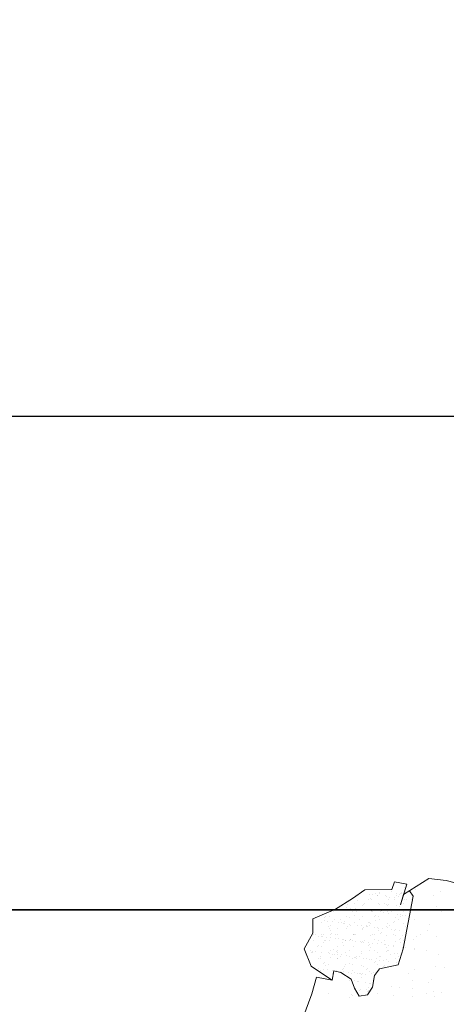
# Model space of a CAD drawing. Units: inches. Extents: x 1986 to 21484, y -1816 to 2016.
# Tile 35 of 85: x 2149 to 2160, y 1898 to 1924. Entities that reach past the tile are written whole.
import ezdxf

# ---------------------------------------------------------------- set-up
doc = ezdxf.new("R2010")
doc.units = ezdxf.units.IN
for name, color, linetype, lineweight in [('A-ANNO-DIMS', 2, 'Continuous', 18), ('C-PROP', 7, 'Continuous', 35), ('L-PLNT', 84, 'Continuous', 13)]:
    doc.layers.add(name, color=color, linetype=linetype, lineweight=lineweight)
doc.styles.get("Standard").update_dxf_attribs({"font": 'arial.ttf'})
doc.dimstyles.new('ISO-25', dxfattribs={"dimtxt": 8, "dimasz": 2.5, "dimexe": 1.25, "dimexo": 0.625, "dimtad": 1, "dimdec": 1, "dimlunit": 3, "dimtxsty": 'Standard', "dimcen": 2.5, "dimadec": 0, "dimazin": 0, "dimtfac": 1, "dimtdec": 1, "dimtmove": 0, "dimatfit": 3, "dimfxl": 1, "dimarcsym": 0})

# ---------------------------------------------------------------- blocks, each defined once
blk = doc.blocks.new('*D1')
at = {"layer": 'A-ANNO-DIMS', "color": 0, "lineweight": -2, "transparency": 16777216}
for p, q in [((2042.312, 1901.377), (2042.312, 1914.655)), ((2402.312, 1901.377), (2402.312, 1914.655)), ((2044.812, 1913.405), (2399.812, 1913.405))]:
    blk.add_line(p, q, dxfattribs=at)
at = {"layer": 'A-ANNO-DIMS', "color": 0, "transparency": 16777216}
for points in [[(2044.812, 1913.821), (2044.812, 1912.988), (2042.312, 1913.405)], [(2399.812, 1913.821), (2399.812, 1912.988), (2402.312, 1913.405)]]:
    blk.add_solid(points, dxfattribs=at)
at = {"layer": 'Defpoints', "color": 0, "transparency": 16777216}
for p in [(2402.312, 1913.405), (2042.312, 1900.752), (2402.312, 1900.752)]:
    blk.add_point(p, dxfattribs=at)
at = {"layer": 'A-ANNO-DIMS', "color": 0, "transparency": 16777216, "insert": (2222.312, 1918.117), "char_height": 8, "attachment_point": 5}
blk.add_mtext("30'", dxfattribs=at)
blk = doc.blocks.new('PLANT-SHRUB')
for p, q in [((2158.177, 1901.273), (2158.24, 1901.471)), ((2158.24, 1901.471), (2158.553, 1901.409)), ((2158.553, 1901.409), (2158.396, 1900.877)), ((2158.474, 1901.143), (2159.119, 1901.558)), ((2159.119, 1901.558), (2159.568, 1901.506)), ((2159.119, 1901.558), (2159.119, 1901.558)), ((2159.568, 1901.506), (2159.797, 1901.443)), ((2157.165, 1901.044), (2157.478, 1901.263)), ((2157.478, 1901.263), (2158.177, 1901.273)), ((2157.753, 1901.169), (2157.753, 1901.169)), ((2157.862, 1901.187), (2157.862, 1901.187)), ((2157.862, 1901.159), (2157.862, 1901.159)), ((2158.166, 1901.222), (2158.166, 1901.222)), ((2158.294, 1901.171), (2158.294, 1901.171)), ((2158.36, 1901.158), (2158.36, 1901.158)), ((2158.393, 1901.174), (2158.393, 1901.174)), ((2158.412, 1901.172), (2158.412, 1901.172)), ((2158.423, 1901.201), (2158.423, 1901.201)), ((2158.497, 1901.332), (2158.497, 1901.332)), ((2158.716, 1901.103), (2158.627, 1901.241)), ((2158.791, 1901.264), (2158.791, 1901.264)), ((2159.411, 1901.22), (2159.411, 1901.22)), ((2156.726, 1900.772), (2157.165, 1901.044)), ((2156.98, 1900.915), (2156.98, 1900.915)), ((2157.204, 1900.902), (2157.204, 1900.902)), ((2157.285, 1900.982), (2157.285, 1900.982)), ((2157.478, 1900.914), (2157.478, 1900.914)), ((2157.585, 1901.014), (2157.585, 1901.014)), ((2157.596, 1901.148), (2157.596, 1901.148)), ((2157.614, 1901.041), (2157.614, 1901.041)), ((2157.659, 1901.027), (2157.659, 1901.027)), ((2157.679, 1901.137), (2157.679, 1901.137)), ((2157.795, 1901.116), (2157.795, 1901.116)), ((2157.809, 1901.12), (2157.809, 1901.12)), ((2157.828, 1900.91), (2157.828, 1900.91)), ((2157.976, 1900.913), (2157.976, 1900.913)), ((2157.998, 1901.115), (2157.998, 1901.115)), ((2158.026, 1901.091), (2158.026, 1901.091)), ((2158.078, 1901.022), (2158.078, 1901.022)), ((2158.11, 1901.08), (2158.11, 1901.08)), ((2158.234, 1901.028), (2158.234, 1901.028)), ((2158.24, 1901.063), (2158.24, 1901.063)), ((2158.293, 1901.115), (2158.293, 1901.115)), ((2158.338, 1901.104), (2158.338, 1901.104)), ((2158.396, 1900.877), (2158.474, 1901.143)), ((2158.457, 1901.035), (2158.457, 1901.035)), ((2158.46, 1899.75), (2158.716, 1901.103)), ((2158.474, 1900.912), (2158.474, 1900.912)), ((2158.487, 1901.024), (2158.487, 1901.024)), ((2158.54, 1901.024), (2158.54, 1901.024)), ((2158.67, 1901.007), (2158.67, 1901.007)), ((2159.242, 1901.112), (2159.242, 1901.112)), ((2156.152, 1900.522), (2156.726, 1900.772)), ((2156.617, 1900.709), (2156.617, 1900.709)), ((2156.67, 1900.717), (2156.67, 1900.717)), ((2156.737, 1900.76), (2156.737, 1900.76)), ((2156.808, 1900.732), (2156.808, 1900.732)), ((2157.018, 1900.81), (2157.018, 1900.81)), ((2157.025, 1900.882), (2157.025, 1900.882)), ((2157.102, 1900.799), (2157.102, 1900.799)), ((2157.168, 1900.716), (2157.168, 1900.716)), ((2157.217, 1900.734), (2157.217, 1900.734)), ((2157.231, 1900.782), (2157.231, 1900.782)), ((2157.235, 1900.759), (2157.235, 1900.759)), ((2157.257, 1900.714), (2157.257, 1900.714)), ((2157.287, 1900.741), (2157.287, 1900.741)), ((2157.426, 1900.868), (2157.426, 1900.868)), ((2157.443, 1900.877), (2157.443, 1900.877)), ((2157.449, 1900.753), (2157.449, 1900.753)), ((2157.532, 1900.742), (2157.532, 1900.742)), ((2157.649, 1900.719), (2157.649, 1900.719)), ((2157.662, 1900.725), (2157.662, 1900.725)), ((2157.666, 1900.715), (2157.666, 1900.715)), ((2157.733, 1900.758), (2157.733, 1900.758)), ((2157.852, 1900.879), (2157.852, 1900.879)), ((2157.879, 1900.697), (2157.879, 1900.697)), ((2157.906, 1900.728), (2157.906, 1900.728)), ((2157.941, 1900.74), (2157.941, 1900.74)), ((2157.962, 1900.686), (2157.962, 1900.686)), ((2158.036, 1900.883), (2158.036, 1900.883)), ((2158.065, 1900.874), (2158.065, 1900.874)), ((2158.068, 1900.714), (2158.068, 1900.714)), ((2158.092, 1900.669), (2158.092, 1900.669)), ((2158.095, 1900.901), (2158.095, 1900.901)), ((2158.163, 1900.714), (2158.163, 1900.714)), ((2158.231, 1900.757), (2158.231, 1900.757)), ((2158.284, 1900.863), (2158.284, 1900.863)), ((2158.284, 1900.863), (2158.284, 1900.863)), ((2158.361, 1900.84), (2158.361, 1900.84)), ((2158.477, 1900.715), (2158.477, 1900.715)), ((2158.546, 1900.734), (2158.546, 1900.734)), ((2158.575, 1900.761), (2158.575, 1900.761)), ((2158.904, 1900.769), (2158.904, 1900.769)), ((2159.112, 1900.741), (2159.112, 1900.741)), ((2159.33, 1900.85), (2159.33, 1900.85)), ((2159.437, 1900.699), (2159.437, 1900.699)), ((2159.54, 1900.753), (2159.54, 1900.753)), ((2156.152, 1900.157), (2156.152, 1900.522)), ((2156.38, 1900.43), (2156.38, 1900.43)), ((2156.441, 1900.472), (2156.441, 1900.472)), ((2156.449, 1900.554), (2156.449, 1900.554)), ((2156.478, 1900.581), (2156.478, 1900.581)), ((2156.524, 1900.461), (2156.524, 1900.461)), ((2156.583, 1900.59), (2156.583, 1900.59)), ((2156.654, 1900.444), (2156.654, 1900.444)), ((2156.697, 1900.502), (2156.697, 1900.502)), ((2156.798, 1900.424), (2156.798, 1900.424)), ((2156.851, 1900.514), (2156.851, 1900.514)), ((2156.871, 1900.416), (2156.871, 1900.416)), ((2156.929, 1900.414), (2156.929, 1900.414)), ((2156.954, 1900.405), (2156.954, 1900.405)), ((2156.959, 1900.441), (2156.959, 1900.441)), ((2157.014, 1900.574), (2157.014, 1900.574)), ((2157.098, 1900.568), (2157.098, 1900.568)), ((2157.206, 1900.61), (2157.206, 1900.61)), ((2157.207, 1900.426), (2157.207, 1900.426)), ((2157.349, 1900.513), (2157.349, 1900.513)), ((2157.433, 1900.569), (2157.433, 1900.569)), ((2157.579, 1900.428), (2157.579, 1900.428)), ((2157.593, 1900.421), (2157.593, 1900.421)), ((2157.639, 1900.411), (2157.639, 1900.411)), ((2157.738, 1900.574), (2157.738, 1900.574)), ((2157.743, 1900.489), (2157.743, 1900.489)), ((2157.767, 1900.601), (2157.767, 1900.601)), ((2157.842, 1900.571), (2157.842, 1900.571)), ((2157.847, 1900.513), (2157.847, 1900.513)), ((2158.057, 1900.405), (2158.057, 1900.405)), ((2158.218, 1900.433), (2158.218, 1900.433)), ((2158.248, 1900.46), (2158.248, 1900.46)), ((2158.274, 1900.555), (2158.274, 1900.555)), ((2158.309, 1900.64), (2158.309, 1900.64)), ((2158.344, 1900.512), (2158.344, 1900.512)), ((2158.387, 1900.588), (2158.387, 1900.588)), ((2158.392, 1900.629), (2158.392, 1900.629)), ((2158.45, 1900.608), (2158.45, 1900.608)), ((2158.466, 1900.407), (2158.466, 1900.407)), ((2158.522, 1900.612), (2158.522, 1900.612)), ((2158.766, 1900.494), (2158.766, 1900.494)), ((2155.923, 1899.751), (2156.152, 1900.157)), ((2156.541, 1900.317), (2156.541, 1900.317)), ((2156.573, 1900.282), (2156.573, 1900.282)), ((2156.599, 1900.224), (2156.599, 1900.224)), ((2156.608, 1900.36), (2156.608, 1900.36)), ((2156.77, 1900.268), (2156.77, 1900.268)), ((2157.004, 1900.266), (2157.004, 1900.266)), ((2157.039, 1900.316), (2157.039, 1900.316)), ((2157.084, 1900.388), (2157.084, 1900.388)), ((2157.106, 1900.359), (2157.106, 1900.359)), ((2157.301, 1900.359), (2157.301, 1900.359)), ((2157.384, 1900.348), (2157.384, 1900.348)), ((2157.41, 1900.273), (2157.41, 1900.273)), ((2157.423, 1900.261), (2157.423, 1900.261)), ((2157.44, 1900.3), (2157.44, 1900.3)), ((2157.514, 1900.331), (2157.514, 1900.331)), ((2157.519, 1900.353), (2157.519, 1900.353)), ((2157.537, 1900.315), (2157.537, 1900.315)), ((2157.604, 1900.358), (2157.604, 1900.358)), ((2157.732, 1900.302), (2157.732, 1900.302)), ((2157.815, 1900.291), (2157.815, 1900.291)), ((2157.832, 1900.263), (2157.832, 1900.263)), ((2157.843, 1900.221), (2157.843, 1900.221)), ((2157.92, 1900.16), (2157.92, 1900.16)), ((2157.945, 1900.274), (2157.945, 1900.274)), ((2158.034, 1900.314), (2158.034, 1900.314)), ((2158.059, 1900.288), (2158.059, 1900.288)), ((2158.102, 1900.357), (2158.102, 1900.357)), ((2158.162, 1900.246), (2158.162, 1900.246)), ((2158.245, 1900.235), (2158.245, 1900.235)), ((2158.264, 1900.247), (2158.264, 1900.247)), ((2158.375, 1900.218), (2158.375, 1900.218)), ((2158.532, 1900.313), (2158.532, 1900.313)), ((2159.088, 1900.219), (2159.088, 1900.219)), ((2159.142, 1900.389), (2159.142, 1900.389)), ((2156.154, 1899.972), (2156.154, 1899.972)), ((2156.157, 1900.127), (2156.157, 1900.127)), ((2156.224, 1900.115), (2156.224, 1900.115)), ((2156.293, 1900.078), (2156.293, 1900.078)), ((2156.37, 1900.122), (2156.37, 1900.122)), ((2156.376, 1900.067), (2156.376, 1900.067)), ((2156.384, 1900.066), (2156.384, 1900.066)), ((2156.412, 1899.916), (2156.412, 1899.916)), ((2156.43, 1900.116), (2156.43, 1900.116)), ((2156.443, 1899.968), (2156.443, 1899.968)), ((2156.479, 1899.959), (2156.479, 1899.959)), ((2156.506, 1900.05), (2156.506, 1900.05)), ((2156.563, 1899.974), (2156.563, 1899.974)), ((2156.592, 1900.038), (2156.592, 1900.038)), ((2156.602, 1900.114), (2156.602, 1900.114)), ((2156.631, 1900.141), (2156.631, 1900.141)), ((2156.722, 1900.114), (2156.722, 1900.114)), ((2156.723, 1900.021), (2156.723, 1900.021)), ((2156.788, 1900.116), (2156.788, 1900.116)), ((2156.807, 1900.01), (2156.807, 1900.01)), ((2156.91, 1899.916), (2156.91, 1899.916)), ((2156.916, 1899.996), (2156.916, 1899.996)), ((2156.937, 1899.993), (2156.937, 1899.993)), ((2156.977, 1899.958), (2156.977, 1899.958)), ((2156.994, 1899.958), (2156.994, 1899.958)), ((2157.082, 1899.973), (2157.082, 1899.973)), ((2157.112, 1900), (2157.112, 1900)), ((2157.121, 1899.989), (2157.121, 1899.989)), ((2157.154, 1899.964), (2157.154, 1899.964)), ((2157.179, 1900.132), (2157.179, 1900.132)), ((2157.197, 1900.118), (2157.197, 1900.118)), ((2157.22, 1900.113), (2157.22, 1900.113)), ((2157.237, 1899.953), (2157.237, 1899.953)), ((2157.251, 1900.128), (2157.251, 1900.128)), ((2157.367, 1899.936), (2157.367, 1899.936)), ((2157.407, 1899.915), (2157.407, 1899.915)), ((2157.413, 1899.953), (2157.413, 1899.953)), ((2157.459, 1899.924), (2157.459, 1899.924)), ((2157.475, 1899.958), (2157.475, 1899.958)), ((2157.584, 1899.908), (2157.584, 1899.908)), ((2157.629, 1900.103), (2157.629, 1900.103)), ((2157.667, 1899.897), (2157.667, 1899.897)), ((2157.667, 1899.897), (2157.667, 1899.897)), ((2157.675, 1900.114), (2157.675, 1900.114)), ((2157.718, 1900.112), (2157.718, 1900.112)), ((2157.732, 1899.987), (2157.732, 1899.987)), ((2157.822, 1899.955), (2157.822, 1899.955)), ((2157.891, 1900.133), (2157.891, 1900.133)), ((2157.905, 1899.914), (2157.905, 1899.914)), ((2157.973, 1899.957), (2157.973, 1899.957)), ((2158.047, 1900.097), (2158.047, 1900.097)), ((2158.215, 1900.111), (2158.215, 1900.111)), ((2158.254, 1899.939), (2158.254, 1899.939)), ((2158.259, 1900.093), (2158.259, 1900.093)), ((2158.371, 1899.993), (2158.371, 1899.993)), ((2158.401, 1900.02), (2158.401, 1900.02)), ((2158.403, 1899.913), (2158.403, 1899.913)), ((2158.456, 1900.099), (2158.456, 1900.099)), ((2158.471, 1899.956), (2158.471, 1899.956)), ((2158.721, 1900.003), (2158.721, 1900.003)), ((2158.794, 1900.07), (2158.794, 1900.07)), ((2158.919, 1900.112), (2158.919, 1900.112)), ((2159.305, 1900.08), (2159.305, 1900.08)), ((2156.102, 1899.305), (2155.923, 1899.751)), ((2156.095, 1899.715), (2156.095, 1899.715)), ((2156.115, 1899.667), (2156.115, 1899.667)), ((2156.143, 1899.664), (2156.143, 1899.664)), ((2156.146, 1899.683), (2156.146, 1899.683)), ((2156.229, 1899.672), (2156.229, 1899.672)), ((2156.274, 1899.813), (2156.274, 1899.813)), ((2156.304, 1899.84), (2156.304, 1899.84)), ((2156.359, 1899.655), (2156.359, 1899.655)), ((2156.36, 1899.814), (2156.36, 1899.814)), ((2156.552, 1899.666), (2156.552, 1899.666)), ((2156.593, 1899.714), (2156.593, 1899.714)), ((2156.672, 1899.732), (2156.672, 1899.732)), ((2156.755, 1899.673), (2156.755, 1899.673)), ((2156.774, 1899.67), (2156.774, 1899.67)), ((2156.778, 1899.808), (2156.778, 1899.808)), ((2156.784, 1899.7), (2156.784, 1899.7)), ((2156.923, 1899.827), (2156.923, 1899.827)), ((2156.984, 1899.65), (2156.984, 1899.65)), ((2157.091, 1899.713), (2157.091, 1899.713)), ((2157.187, 1899.81), (2157.187, 1899.81)), ((2157.403, 1899.645), (2157.403, 1899.645)), ((2157.404, 1899.687), (2157.404, 1899.687)), ((2157.563, 1899.833), (2157.563, 1899.833)), ((2157.588, 1899.712), (2157.588, 1899.712)), ((2157.592, 1899.86), (2157.592, 1899.86)), ((2157.619, 1899.795), (2157.619, 1899.795)), ((2157.718, 1899.719), (2157.718, 1899.719)), ((2157.797, 1899.88), (2157.797, 1899.88)), ((2157.812, 1899.647), (2157.812, 1899.647)), ((2157.992, 1899.854), (2157.992, 1899.854)), ((2158.014, 1899.851), (2158.014, 1899.851)), ((2158.037, 1899.789), (2158.037, 1899.789)), ((2158.044, 1899.693), (2158.044, 1899.693)), ((2158.073, 1899.72), (2158.073, 1899.72)), ((2158.086, 1899.711), (2158.086, 1899.711)), ((2158.098, 1899.84), (2158.098, 1899.84)), ((2158.212, 1899.847), (2158.212, 1899.847)), ((2158.228, 1899.823), (2158.228, 1899.823)), ((2158.332, 1899.345), (2158.46, 1899.75)), ((2158.445, 1899.794), (2158.445, 1899.794)), ((2158.446, 1899.791), (2158.446, 1899.791)), ((2158.535, 1899.783), (2158.535, 1899.783)), ((2158.741, 1899.723), (2158.741, 1899.723)), ((2158.743, 1899.755), (2158.743, 1899.755)), ((2159.068, 1899.712), (2159.068, 1899.712)), ((2156.283, 1899.516), (2156.283, 1899.516)), ((2156.35, 1899.559), (2156.35, 1899.559)), ((2156.35, 1899.506), (2156.35, 1899.506)), ((2156.457, 1899.4), (2156.457, 1899.4)), ((2156.576, 1899.627), (2156.576, 1899.627)), ((2156.596, 1899.527), (2156.596, 1899.527)), ((2156.659, 1899.616), (2156.659, 1899.616)), ((2156.7, 1899.603), (2156.7, 1899.603)), ((2156.768, 1899.5), (2156.768, 1899.5)), ((2156.78, 1899.515), (2156.78, 1899.515)), ((2156.789, 1899.598), (2156.789, 1899.598)), ((2156.848, 1899.558), (2156.848, 1899.558)), ((2156.883, 1899.609), (2156.883, 1899.609)), ((2157.006, 1899.57), (2157.006, 1899.57)), ((2157.09, 1899.559), (2157.09, 1899.559)), ((2157.177, 1899.502), (2157.177, 1899.502)), ((2157.22, 1899.542), (2157.22, 1899.542)), ((2157.235, 1899.533), (2157.235, 1899.533)), ((2157.265, 1899.56), (2157.265, 1899.56)), ((2157.278, 1899.514), (2157.278, 1899.514)), ((2157.346, 1899.557), (2157.346, 1899.557)), ((2157.437, 1899.513), (2157.437, 1899.513)), ((2157.52, 1899.502), (2157.52, 1899.502)), ((2157.609, 1899.487), (2157.609, 1899.487)), ((2157.65, 1899.485), (2157.65, 1899.485)), ((2157.716, 1899.392), (2157.716, 1899.392)), ((2157.745, 1899.419), (2157.745, 1899.419)), ((2157.776, 1899.513), (2157.776, 1899.513)), ((2157.844, 1899.556), (2157.844, 1899.556)), ((2157.867, 1899.457), (2157.867, 1899.457)), ((2157.884, 1899.547), (2157.884, 1899.547)), ((2157.95, 1899.446), (2157.95, 1899.446)), ((2158.027, 1899.481), (2158.027, 1899.481)), ((2158.08, 1899.429), (2158.08, 1899.429)), ((2158.127, 1899.607), (2158.127, 1899.607)), ((2158.243, 1899.631), (2158.243, 1899.631)), ((2158.274, 1899.512), (2158.274, 1899.512)), ((2158.297, 1899.4), (2158.297, 1899.4)), ((2158.323, 1899.638), (2158.323, 1899.638)), ((2158.341, 1899.555), (2158.341, 1899.555)), ((2159.372, 1899.605), (2159.372, 1899.605)), ((2156.162, 1899.266), (2156.102, 1899.305)), ((2156.642, 1898.953), (2156.162, 1899.266)), ((2156.302, 1899.238), (2156.302, 1899.238)), ((2156.34, 1899.198), (2156.34, 1899.198)), ((2156.427, 1899.373), (2156.427, 1899.373)), ((2156.429, 1899.232), (2156.429, 1899.232)), ((2156.464, 1899.313), (2156.464, 1899.313)), ((2156.512, 1899.221), (2156.512, 1899.221)), ((2156.542, 1899.358), (2156.542, 1899.358)), ((2156.642, 1899.204), (2156.642, 1899.204)), ((2156.642, 1898.953), (2156.685, 1899.186)), ((2156.685, 1899.186), (2156.865, 1899.149)), ((2156.758, 1899.192), (2156.758, 1899.192)), ((2156.859, 1899.175), (2156.859, 1899.175)), ((2156.865, 1899.149), (2157.131, 1898.976)), ((2156.908, 1899.232), (2156.908, 1899.232)), ((2156.937, 1899.259), (2156.937, 1899.259)), ((2156.942, 1899.164), (2156.942, 1899.164)), ((2156.961, 1899.312), (2156.961, 1899.312)), ((2156.974, 1899.342), (2156.974, 1899.342)), ((2157.072, 1899.147), (2157.072, 1899.147)), ((2157.076, 1899.387), (2157.076, 1899.387)), ((2157.154, 1899.362), (2157.154, 1899.362)), ((2157.167, 1899.194), (2157.167, 1899.194)), ((2157.217, 1899.157), (2157.217, 1899.157)), ((2157.393, 1899.337), (2157.393, 1899.337)), ((2157.459, 1899.312), (2157.459, 1899.312)), ((2157.521, 1899.22), (2157.521, 1899.22)), ((2157.557, 1899.247), (2157.557, 1899.247)), ((2157.599, 1899.179), (2157.599, 1899.179)), ((2157.714, 1899.156), (2157.714, 1899.156)), ((2157.732, 1899.068), (2157.859, 1899.242)), ((2157.802, 1899.339), (2157.802, 1899.339)), ((2157.859, 1899.242), (2158.332, 1899.345)), ((2157.902, 1899.252), (2157.902, 1899.252)), ((2157.957, 1899.311), (2157.957, 1899.311)), ((2157.975, 1899.32), (2157.975, 1899.32)), ((2158.233, 1899.323), (2158.233, 1899.323)), ((2158.332, 1899.345), (2158.332, 1899.345)), ((2158.765, 1899.218), (2158.765, 1899.218)), ((2159.28, 1899.31), (2159.28, 1899.31)), ((2159.524, 1899.287), (2159.524, 1899.287)), ((2156.12, 1898.599), (2156.245, 1899.026)), ((2156.245, 1899.026), (2156.642, 1898.953)), ((2156.647, 1898.962), (2156.647, 1898.962)), ((2156.651, 1899.115), (2156.651, 1899.115)), ((2157.091, 1898.938), (2157.091, 1898.938)), ((2157.131, 1898.976), (2157.212, 1898.745)), ((2157.149, 1899.114), (2157.149, 1899.114)), ((2157.229, 1898.946), (2157.229, 1898.946)), ((2157.289, 1899.119), (2157.289, 1899.119)), ((2157.299, 1898.911), (2157.299, 1898.911)), ((2157.33, 1898.911), (2157.33, 1898.911)), ((2157.352, 1899.113), (2157.352, 1899.113)), ((2157.373, 1899.108), (2157.373, 1899.108)), ((2157.383, 1899.029), (2157.383, 1899.029)), ((2157.388, 1899.092), (2157.388, 1899.092)), ((2157.418, 1899.119), (2157.418, 1899.119)), ((2157.503, 1899.091), (2157.503, 1899.091)), ((2157.504, 1898.888), (2157.504, 1898.888)), ((2157.647, 1899.113), (2157.647, 1899.113)), ((2157.674, 1898.768), (2157.732, 1899.068)), ((2157.693, 1898.948), (2157.693, 1898.948)), ((2157.72, 1899.062), (2157.72, 1899.062)), ((2158.597, 1899.111), (2158.597, 1899.111)), ((2158.715, 1898.953), (2158.715, 1898.953)), ((2159.103, 1898.901), (2159.103, 1898.901)), ((2159.177, 1898.969), (2159.177, 1898.969)), ((2157.212, 1898.745), (2157.339, 1898.537)), ((2157.355, 1898.696), (2157.355, 1898.696)), ((2157.372, 1898.721), (2157.372, 1898.721)), ((2157.518, 1898.713), (2157.518, 1898.713)), ((2157.541, 1898.652), (2157.541, 1898.652)), ((2157.547, 1898.572), (2157.674, 1898.768)), ((2157.571, 1898.679), (2157.571, 1898.679)), ((2157.572, 1898.668), (2157.572, 1898.668)), ((2157.585, 1898.756), (2157.585, 1898.756)), ((2157.589, 1898.871), (2157.589, 1898.871)), ((2157.624, 1898.868), (2157.624, 1898.868)), ((2158.167, 1898.796), (2158.167, 1898.796)), ((2158.375, 1898.769), (2158.375, 1898.769)), ((2158.7, 1898.726), (2158.7, 1898.726)), ((2159.242, 1898.655), (2159.242, 1898.655)), ((2155.89, 1897.973), (2156.12, 1898.599)), ((2156.56, 1898.608), (2156.56, 1898.608)), ((2157.082, 1898.501), (2157.082, 1898.501)), ((2157.129, 1898.592), (2157.129, 1898.592)), ((2157.156, 1898.569), (2157.156, 1898.569)), ((2157.339, 1898.537), (2157.547, 1898.572)), ((2157.805, 1898.606), (2157.805, 1898.606)), ((2158.208, 1898.553), (2158.208, 1898.553)), ((2158.705, 1898.537), (2158.705, 1898.537)), ((2159.049, 1898.604), (2159.049, 1898.604)), ((2159.254, 1898.54), (2159.254, 1898.54)), ((2159.451, 1898.627), (2159.451, 1898.627))]:
    blk.add_line(p, q)

msp = doc.modelspace()

# ---------------------------------------------------------------- linework, layer by layer
at = {"layer": 'C-PROP'}
msp.add_lwpolyline([(2042.312, 1900.752), (2402.312, 1900.752), (2402.312, 1066.752), (2042.312, 1066.752)], close=True, dxfattribs=at)

# ---------------------------------------------------------------- block references
at = {"layer": 'L-PLNT'}
msp.add_blockref('PLANT-SHRUB', (0, 0), dxfattribs=at)

# ---------------------------------------------------------------- dimensions: what is measured, and where the dimension line sits
at = {"layer": 'A-ANNO-DIMS'}
dim = msp.add_linear_dim(base=(2402.312, 1913.405), p1=(2042.312, 1900.752), p2=(2402.312, 1900.752), dimstyle='ISO-25', override={"dimclrd": 0, "dimclre": 0, "dimclrt": 0}, dxfattribs=at)
dim.commit()
dim.dimension.update_dxf_attribs({"geometry": '*D1', "text_midpoint": (2222.312, 1918.117)})

doc.saveas('drawing.dxf')
